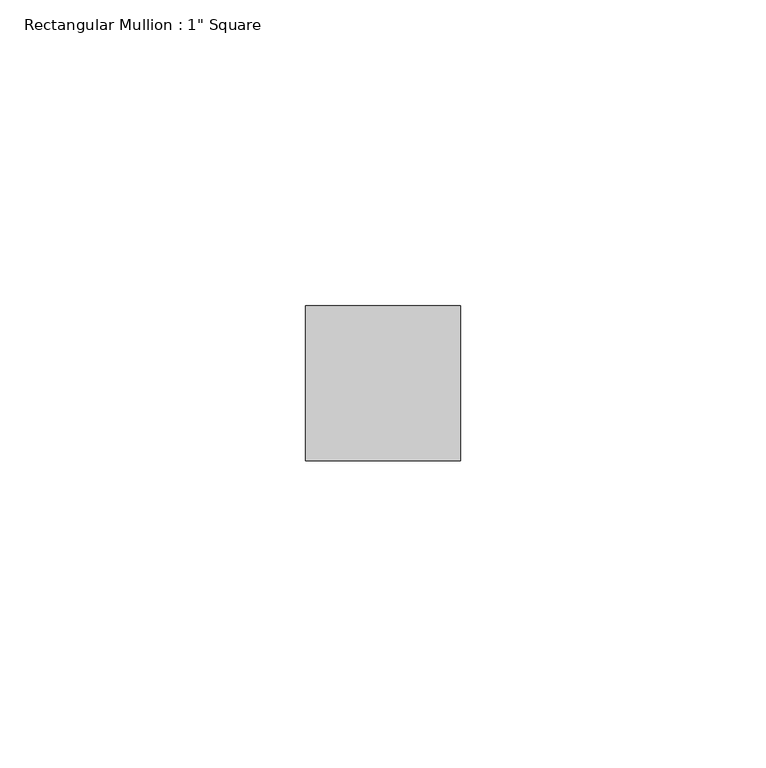
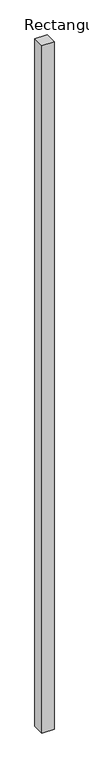
"""IFC4 building model written with IfcOpenShell, lengths in millimetres: member geometry."""

from ifc_helpers import new_model, si_unit, frame, origin, place, context, project, spatial, polyline, outline, extrude, source, transform, mapped, element, save


def member_d76f7ec7(model_context):
    return source(origin(), model_context, "Body", "SweptSolid", [
        extrude(outline(polyline([(0.0, 12.7), (0.0, -12.7), (-25.4, -12.7), (-25.4, 12.7), (0.0, 12.7)])), frame((0.0, 0.0, -1524.0), z_axis=(0.0, 0.0, 1.0), x_axis=(1.0, 0.0, 0.0)), (0.0, 0.0, 1.0), 1524.0),
    ])


if __name__ == "__main__":
    model = new_model("IFC4")
    model_context = context("Model", 3, world=origin())
    ifc_project = project(units=[si_unit("LENGTHUNIT", "METRE", prefix="MILLI")], contexts=[model_context])
    site = spatial("IfcSite", under=ifc_project)
    building = spatial("IfcBuilding", under=site)
    placement = place(None, origin())
    member_shape = member_d76f7ec7(model_context)
    element("IfcMember", 1, ObjectType="Rectangular Mullion : 1\" Square", at=placement, inside=building, context=model_context, shape_type="MappedRepresentation", body=[
        mapped(member_shape, transform((0.0, 0.0, 0.0), x_axis=(1.0, 0.0, 0.0), y_axis=(0.0, 1.0, 0.0), z_axis=(0.0, 0.0, 1.0))),
    ])
    save(model, "model.ifc")

# Revit data of these elements
# Type "Rectangular Mullion : 1\" Square"
#   built-in parameter 1007304 = 0.0833333 (stored number, unit not read)
#   built-in parameter 1007301 = 0.0416667 (stored number, unit not read)
#   built-in parameter 1007300 = 0.0416667 (stored number, unit not read)
